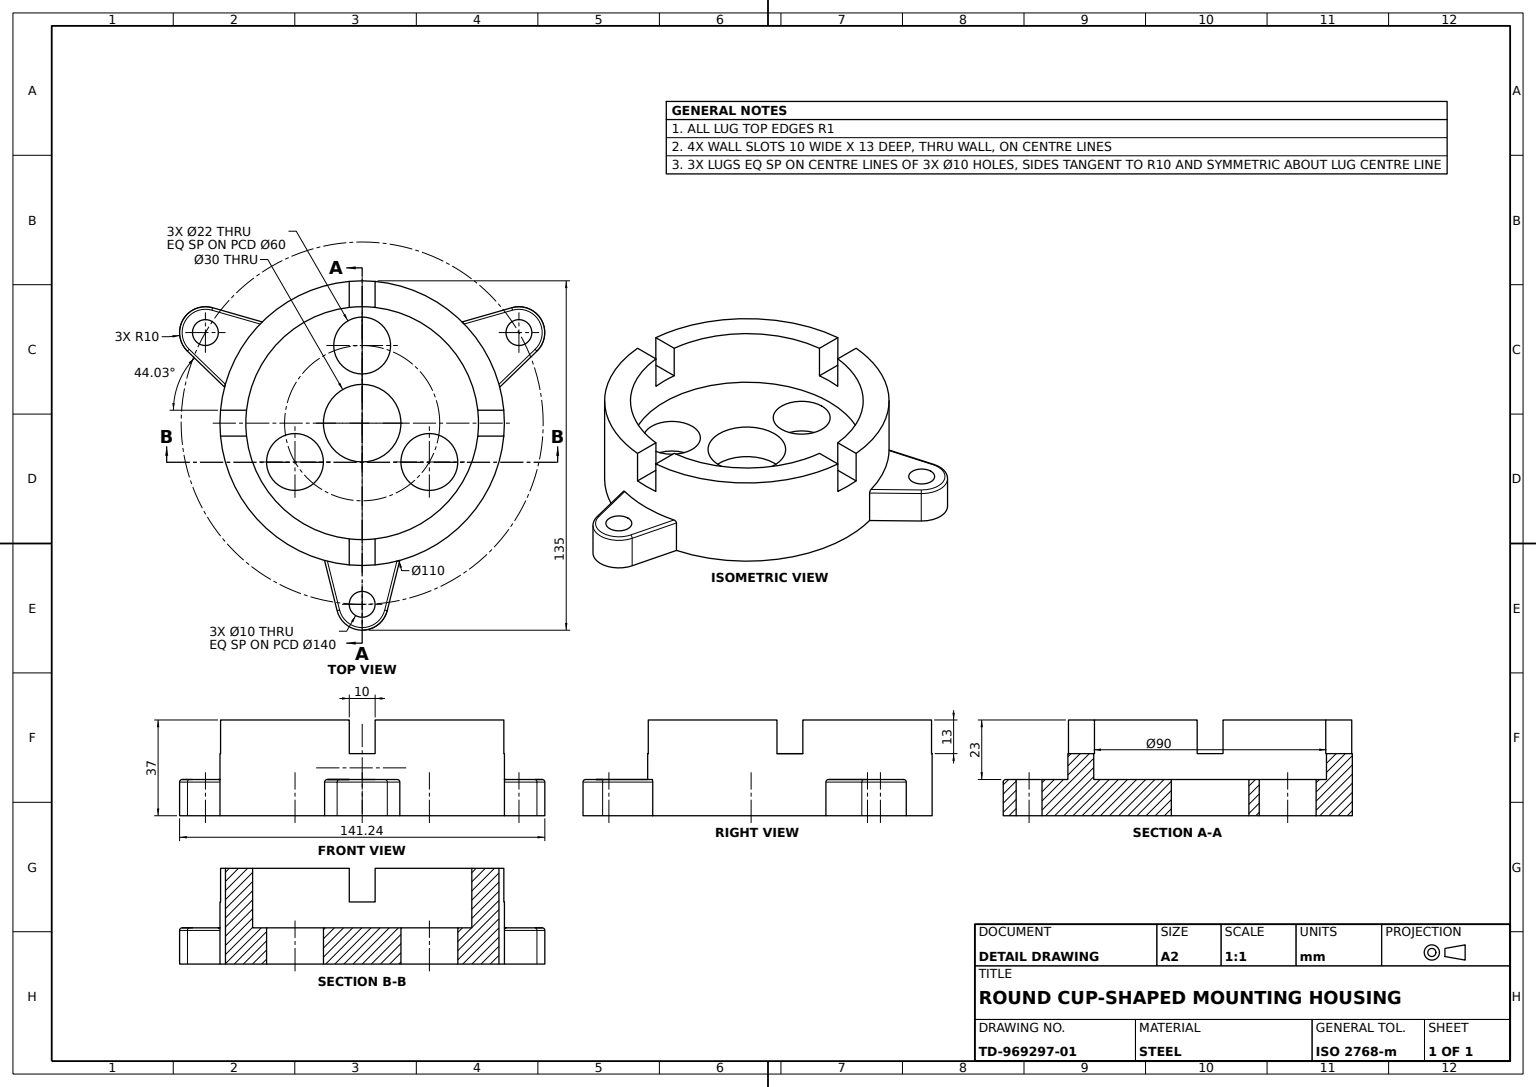
from build123d import *

# Parameters (mm, degrees)
FLANGE_PROFILE_SKETCH_R      = 45
FLANGE_PROFILE_SKETCH_R_2    = 5
FLANGE_PROFILE_SKETCH_R_3    = 15
FLANGE_PROFILE_SKETCH_R_4    = 11
MOUNTING_FLANGE_3_LUGS_DEPTH = 14
FLANGE_EDGE_FILLET_R1_R      = 1
BEARING_WALL_SKETCH_R        = 55
BEARING_WALL_SKETCH_R_2      = 45
BEARING_WALL_110_DEPTH       = 23
WALL_START                   = -13
WALL_SLOTS_4X_DEPTH          = 13


with BuildPart() as part:
    # Flange Profile Sketch → Mounting Flange 3 Lugs (new body)
    # profile 1 of 2: a face of its own
    with BuildSketch(Plane(origin=(0, 0, 0), x_dir=(1, 0, 0), z_dir=(0, 1, 0))):
        with BuildLine():
            Line((9.701823617, -72.423761231), (14.543823193, -53.042220984))
            ThreePointArc((14.543823193, -53.042220984), (47.631397208, -27.5), (53.207822442, 13.925790139))
            Line((53.207822442, 13.925790139), (67.571728872, 27.8098549))
            ThreePointArc((67.571728872, 27.8098549), (69.282032303, 40), (57.869905255, 44.613906331))
            Line((57.869905255, 44.613906331), (38.663999249, 39.116430845))
            ThreePointArc((38.663999249, 39.116430845), (0, 55), (-38.663999249, 39.116430845))
            Line((-38.663999249, 39.116430845), (-57.869905255, 44.613906331))
            ThreePointArc((-57.869905255, 44.613906331), (-69.282032303, 40), (-67.571728872, 27.8098549))
            Line((-67.571728872, 27.8098549), (-53.207822442, 13.925790139))
            ThreePointArc((-53.207822442, 13.925790139), (-47.631397208, -27.5), (-14.543823193, -53.042220984))
            Line((-14.543823193, -53.042220984), (-9.701823617, -72.423761231))
            ThreePointArc((-9.701823617, -72.423761231), (0, -80), (9.701823617, -72.423761231))
        make_face()
        Circle(FLANGE_PROFILE_SKETCH_R, mode=Mode.SUBTRACT)
        with Locations(Location((0, -70, 0), (0, 0, 270))):
            Circle(FLANGE_PROFILE_SKETCH_R_2, mode=Mode.SUBTRACT)
        with Locations(Location((-60.621778265, 35, 0), (0, 0, 270))):
            Circle(FLANGE_PROFILE_SKETCH_R_2, mode=Mode.SUBTRACT)
        with Locations(Location((60.621778265, 35, 0), (0, 0, 270))):
            Circle(FLANGE_PROFILE_SKETCH_R_2, mode=Mode.SUBTRACT)
    # profile 2 of 2: a face of its own
    with BuildSketch(Plane(origin=(0, 0, 0), x_dir=(1, 0, 0), z_dir=(0, 1, 0))):
        Circle(FLANGE_PROFILE_SKETCH_R)
        with Locations(Location((0, 0, 0), (0, 0, 270))):
            Circle(FLANGE_PROFILE_SKETCH_R_3, mode=Mode.SUBTRACT)
        with Locations(Location((-25.980762114, -15, 0), (0, 0, 270))):
            Circle(FLANGE_PROFILE_SKETCH_R_4, mode=Mode.SUBTRACT)
        with Locations(Location((25.980762114, -15, 0), (0, 0, 270))):
            Circle(FLANGE_PROFILE_SKETCH_R_4, mode=Mode.SUBTRACT)
        with Locations(Location((0, 30, 0), (0, 0, 270))):
            Circle(FLANGE_PROFILE_SKETCH_R_4, mode=Mode.SUBTRACT)
    extrude(amount=MOUNTING_FLANGE_3_LUGS_DEPTH)

    # Flange Edge Fillet R1
    flange_edge_fillet_r1_edges = [part.edges().sort_by_distance(p)[0] for p in [
        (12.122823405, 14, 62.732991107),
        (60.389775657, 14, -20.867822519),
        (69.282032303, 14, -40),
        (48.266952252, 14, -41.865168588),
        (-48.266952252, 14, -41.865168588),
        (-69.282032303, 14, -40),
        (-60.389775657, 14, -20.867822519),
        (-12.122823405, 14, 62.732991107),
        (0, 14, 80),
    ]]
    fillet(flange_edge_fillet_r1_edges, radius=FLANGE_EDGE_FILLET_R1_R)

    # Bearing Wall Sketch → Bearing Wall Ø110 (add)
    with BuildSketch(Plane(origin=(0, 14, 0), x_dir=(1, 0, 0), z_dir=(0, 1, 0))):
        with Locations(Location((0, 0, 0), (0, 0, 134.666726854))):
            Circle(BEARING_WALL_SKETCH_R)
        with Locations(Location((0, 0, 0), (0, 0, 270))):
            Circle(BEARING_WALL_SKETCH_R_2, mode=Mode.SUBTRACT)
    extrude(amount=BEARING_WALL_110_DEPTH)

    # Wall Slots Sketch → Wall Slots 4x (cut)
    with BuildSketch(Plane(origin=(0, 37, 0), x_dir=(1, 0, 0), z_dir=(0, 1, 0)).offset(WALL_START)):
        with BuildLine():
            ThreePointArc((-44.72135955, -5), (-45, 0), (-44.72135955, 5))
            Line((-44.72135955, 5), (-54.772255751, 5))
            ThreePointArc((-54.772255751, 5), (-55, 0), (-54.772255751, -5))
            Line((-54.772255751, -5), (-44.72135955, -5))
        make_face()
        with BuildLine():
            Line((-5, 54.772255751), (-5, 44.72135955))
            ThreePointArc((-5, 44.72135955), (0, 45), (5, 44.72135955))
            Line((5, 44.72135955), (5, 54.772255751))
            ThreePointArc((5, 54.772255751), (0, 55), (-5, 54.772255751))
        make_face()
        with BuildLine():
            Line((54.772255751, 5), (44.72135955, 5))
            ThreePointArc((44.72135955, 5), (44.930285887, 2.503879016), (45, 0))
            ThreePointArc((45, 0), (44.930285887, -2.503879016), (44.72135955, -5))
            Line((44.72135955, -5), (54.772255751, -5))
            ThreePointArc((54.772255751, -5), (54.943034437, -2.502592028), (55, 0))
            ThreePointArc((55, 0), (54.943034437, 2.502592028), (54.772255751, 5))
        make_face()
        with BuildLine():
            ThreePointArc((5, -44.72135955), (0, -45), (-5, -44.72135955))
            Line((-5, -44.72135955), (-5, -54.772255751))
            ThreePointArc((-5, -54.772255751), (0, -55), (5, -54.772255751))
            Line((5, -54.772255751), (5, -44.72135955))
        make_face()
    extrude(amount=WALL_SLOTS_4X_DEPTH, mode=Mode.SUBTRACT)


solid = part.part
